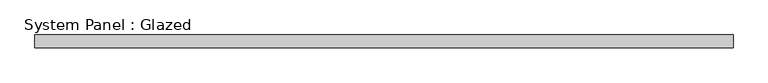
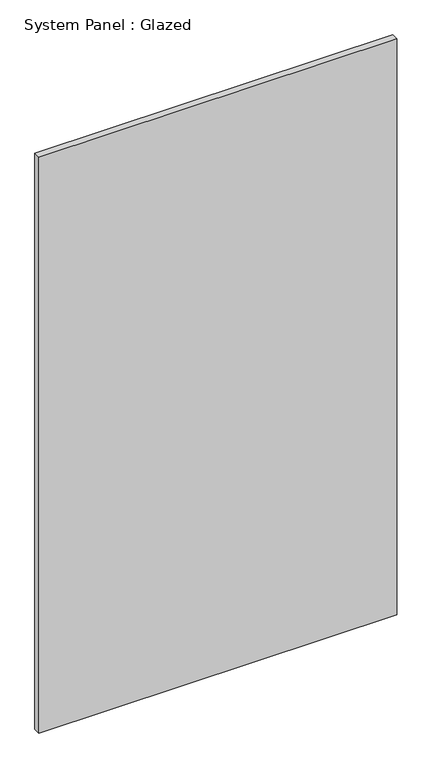
"""IFC4 building model written with IfcOpenShell, lengths in millimetres: plate geometry, System Panel : Glazed."""

from ifc_helpers import new_model, si_unit, origin, origin_with_axes, place, context, project, spatial, polyline, outline, extrude, source, transform, mapped, element, save


def system_panel_glazed_c99c457a(model_context):
    return source(origin(), model_context, "Body", "SweptSolid", [
        extrude(outline(polyline([(688.975, 19.05), (-688.975, 19.05), (-688.975, 44.45), (688.975, 44.45), (688.975, 19.05)])), origin_with_axes(), (0.0, 0.0, 1.0), 2343.15),
    ])


if __name__ == "__main__":
    model = new_model("IFC4")
    model_context = context("Model", 3, world=origin())
    ifc_project = project(units=[si_unit("LENGTHUNIT", "METRE", prefix="MILLI")], contexts=[model_context])
    site = spatial("IfcSite", under=ifc_project)
    building = spatial("IfcBuilding", under=site)
    placement = place(None, origin())
    system_panel_glazed_shape = system_panel_glazed_c99c457a(model_context)
    element("IfcPlate", 1, ObjectType="System Panel : Glazed", at=placement, inside=building, context=model_context, shape_type="MappedRepresentation", body=[
        mapped(system_panel_glazed_shape, transform((0.0, 0.0, 0.0), x_axis=(1.0, 0.0, 0.0), y_axis=(0.0, 1.0, 0.0), z_axis=(0.0, 0.0, 1.0))),
    ])
    save(model, "model.ifc")

# Revit data of these elements
# Type "System Panel : Glazed"
#   Construction Type Id = "GSP4R"
#   Analytic Construction = "1/8 in Pilkington single glazing"
#   Visual Light Transmittance = 0.9
#   Solar Heat Gain Coefficient = 0.86
#   Heat Transfer Coefficient (U) = 1.18115 BTU/(h·ft²·°F)
# Element 1 (IfcPlate, "System Panel : Glazed")
#   Materials on its faces: "Glass"
# Materials
#   "Glass": class "Glass", colour RGB 0 128 192, transparency 0.75, Description = "Soda Lime Glass", Cost = 0
